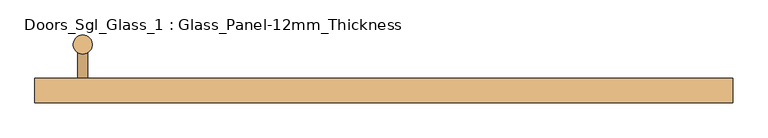
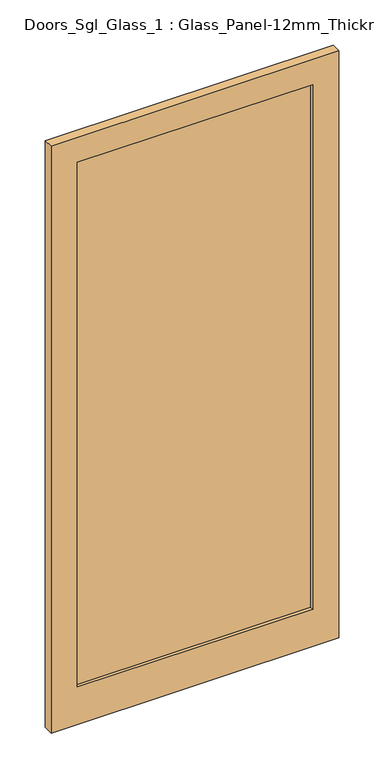
"""IFC4 building model written with IfcOpenShell, lengths in millimetres: door geometry, Doors_Sgl_Glass_1 : Glass_Panel-12mm_Thickness."""

from ifc_helpers import new_model, si_unit, point, frame, frame_2d, origin, place, context, project, spatial, polyline, circle_curve, trimmed, segment, composite_curve, outline, extrude, source, transform, mapped, element, save


def doors_sgl_glass_1_glass_panel_12mm_thickness_3d57b09a(model_context):
    return source(origin(), model_context, "Body", "SweptSolid", [
        extrude(outline(polyline([(446.3031523, 50.0), (446.3031523, 38.0), (-446.3031523, 38.0), (-446.3031523, 50.0), (446.3031523, 50.0)])), frame((0.0, 0.0, 150.0), z_axis=(0.0, 0.0, 1.0), x_axis=(1.0, 0.0, 0.0)), (0.0, 0.0, 1.0), 2105.0),
        extrude(outline(polyline([(0.0, -546.3031523), (0.0, 546.3031523), (2355.0, 546.3031523), (2355.0, -546.3031523), (0.0, -546.3031523)]), holes=[polyline([(2255.0, 446.3031523), (150.0, 446.3031523), (150.0, -446.3031523), (2255.0, -446.3031523), (2255.0, 446.3031523)])]), frame((0.0, 25.0, 0.0), z_axis=(0.0, 1.0, 0.0), x_axis=(0.0, 0.0, 1.0)), (0.0, 0.0, 1.0), 38.0),
        extrude(outline(composite_curve([segment(trimmed(circle_curve(frame_2d((1450.0, -471.3031523)), 8.0), [point((1450.0, -463.3031523))], [point((1450.0, -479.3031523))], False, "CARTESIAN"), True, "CONTINUOUS"), segment(trimmed(circle_curve(frame_2d((1450.0, -471.3031523)), 8.0), [point((1450.0, -479.3031523))], [point((1450.0, -463.3031523))], False, "CARTESIAN"), True, "CONTINUOUS")], self_intersect=False)), frame((0.0, 63.0, 0.0), z_axis=(0.0, 1.0, 0.0), x_axis=(0.0, 0.0, 1.0)), (0.0, 0.0, 1.0), 53.0),
        extrude(outline(composite_curve([segment(trimmed(circle_curve(frame_2d((750.0, -471.3031523)), 8.0), [point((750.0, -463.3031523))], [point((750.0, -479.3031523))], False, "CARTESIAN"), True, "CONTINUOUS"), segment(trimmed(circle_curve(frame_2d((750.0, -471.3031523)), 8.0), [point((750.0, -479.3031523))], [point((750.0, -463.3031523))], False, "CARTESIAN"), True, "CONTINUOUS")], self_intersect=False)), frame((0.0, 63.0, 0.0), z_axis=(0.0, 1.0, 0.0), x_axis=(0.0, 0.0, 1.0)), (0.0, 0.0, 1.0), 53.0),
        extrude(outline(composite_curve([segment(trimmed(circle_curve(frame_2d((-471.3031523, 116.0)), 15.0), [point((-471.3031523, 101.0))], [point((-471.3031523, 131.0))], False, "CARTESIAN"), True, "CONTINUOUS"), segment(trimmed(circle_curve(frame_2d((-471.3031523, 116.0)), 15.0), [point((-471.3031523, 131.0))], [point((-471.3031523, 101.0))], False, "CARTESIAN"), True, "CONTINUOUS")], self_intersect=False)), frame((0.0, 0.0, 650.0), z_axis=(0.0, 0.0, 1.0), x_axis=(1.0, 0.0, 0.0)), (0.0, 0.0, 1.0), 900.0),
    ])


if __name__ == "__main__":
    model = new_model("IFC4")
    model_context = context("Model", 3, world=origin())
    ifc_project = project(units=[si_unit("LENGTHUNIT", "METRE", prefix="MILLI")], contexts=[model_context])
    site = spatial("IfcSite", under=ifc_project)
    building = spatial("IfcBuilding", under=site)
    placement = place(None, origin())
    doors_sgl_glass_1_glass_panel_12mm_thickness_shape = doors_sgl_glass_1_glass_panel_12mm_thickness_3d57b09a(model_context)
    element("IfcDoor", 1, ObjectType="Doors_Sgl_Glass_1 : Glass_Panel-12mm_Thickness", at=placement, inside=building, context=model_context, shape_type="MappedRepresentation", body=[
        mapped(doors_sgl_glass_1_glass_panel_12mm_thickness_shape, transform((0.0, 0.0, 0.0), x_axis=(1.0, 0.0, 0.0), y_axis=(0.0, 1.0, 0.0), z_axis=(0.0, 0.0, 1.0))),
    ])
    save(model, "model.ifc")

# Revit data of these elements
# Type "Doors_Sgl_Glass_1 : Glass_Panel-12mm_Thickness"
#   Type Mark = "60"
#   Construction Type Id = "GSP4R"
#   Keynote = "H11"
#   Analytic Construction = "1/8 in Pilkington single glazing"
#   Visual Light Transmittance = 0.9
#   Stile Top Rail = 0' - 3.93701"
#   Stile Shutting = 0' - 3.93701"
#   Stile Hanging = 0' - 3.93701"
#   Stile Bottom Rail = 0' - 5.90551"
#   Solar Heat Gain Coefficient = 0.78
#   Offset = 0' - 1.9685"
#   Heat Transfer Coefficient (U) = 3.6886 W/(m²·K)
#   Handle X Distance = 0' - 2.95276"
#   Glazing Thickness = 0' - 0.47244"
#   Define Thermal Properties by = 1
#   Material Ironmongery = Metal - Aluminum
#   Material Frame = Metal - Aluminum
#   Material Glass = Glass
#   Function = (empty or 0)
# Element 1 (IfcDoor, "Doors_Sgl_Glass_1 : Glass_Panel-12mm_Thickness")
#   Materials on its faces: "Metal - Aluminum", "Glass"
# Materials
#   "Metal - Aluminum": class "Metal", colour RGB 247 247 247, transparency 0
#   "Glass": class "Glass", colour RGB 0 128 192, transparency 0.9, Description = "Soda Lime Glass", Cost = 0
